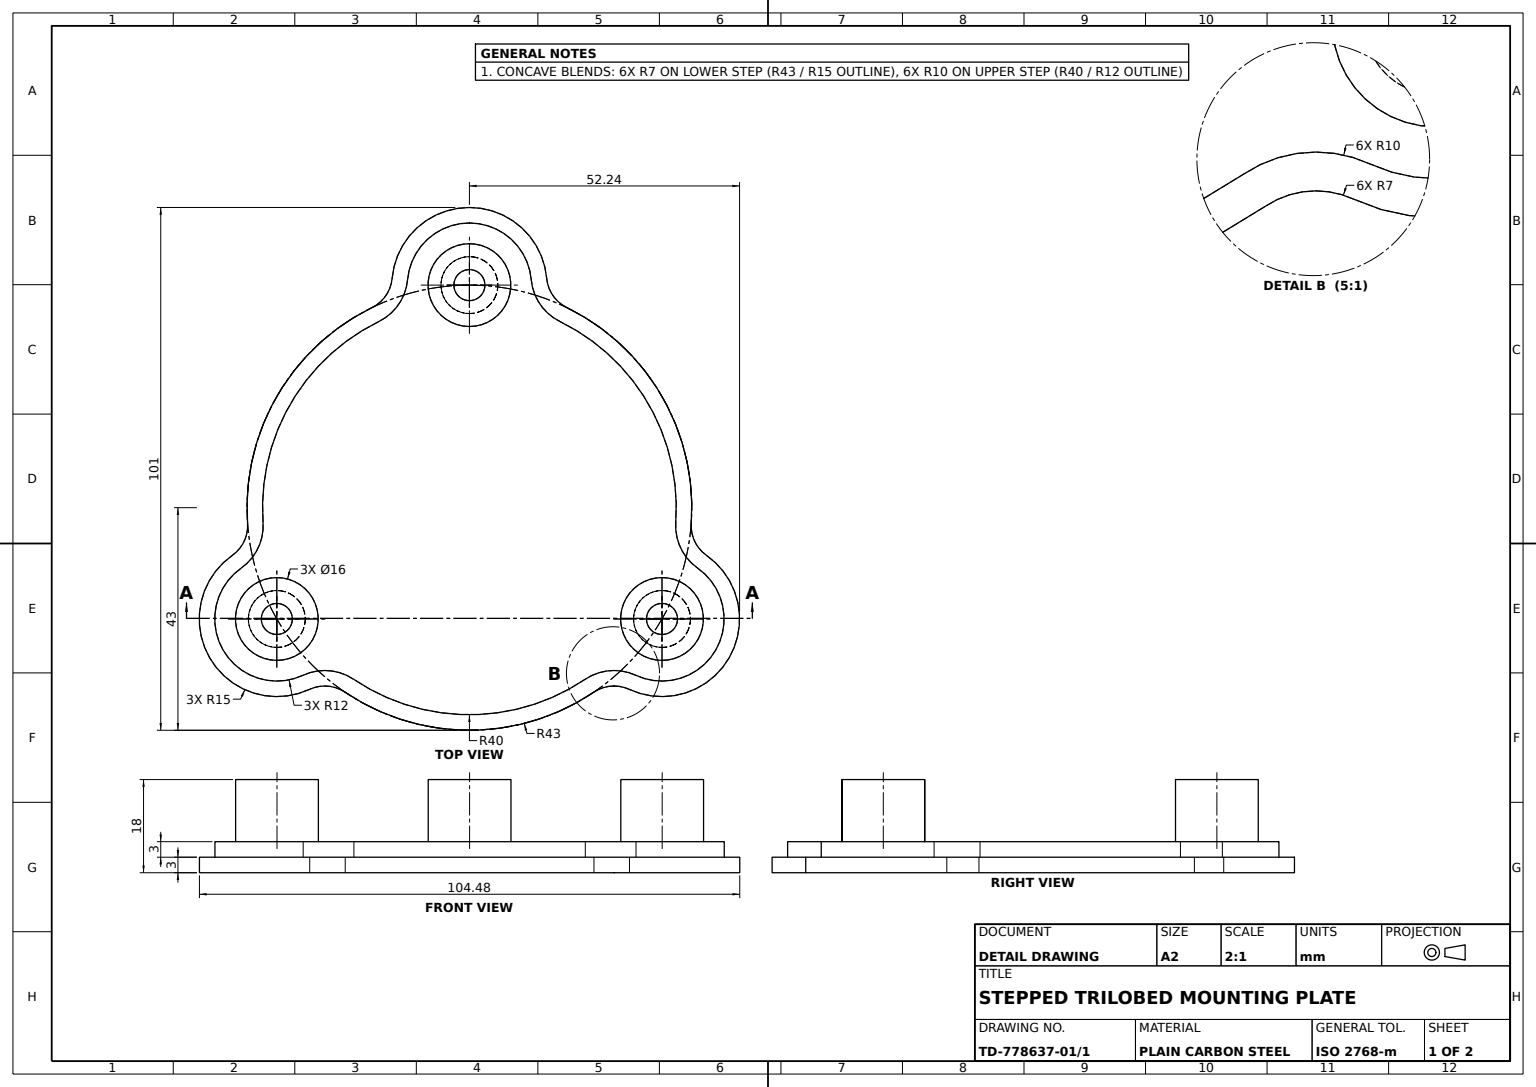
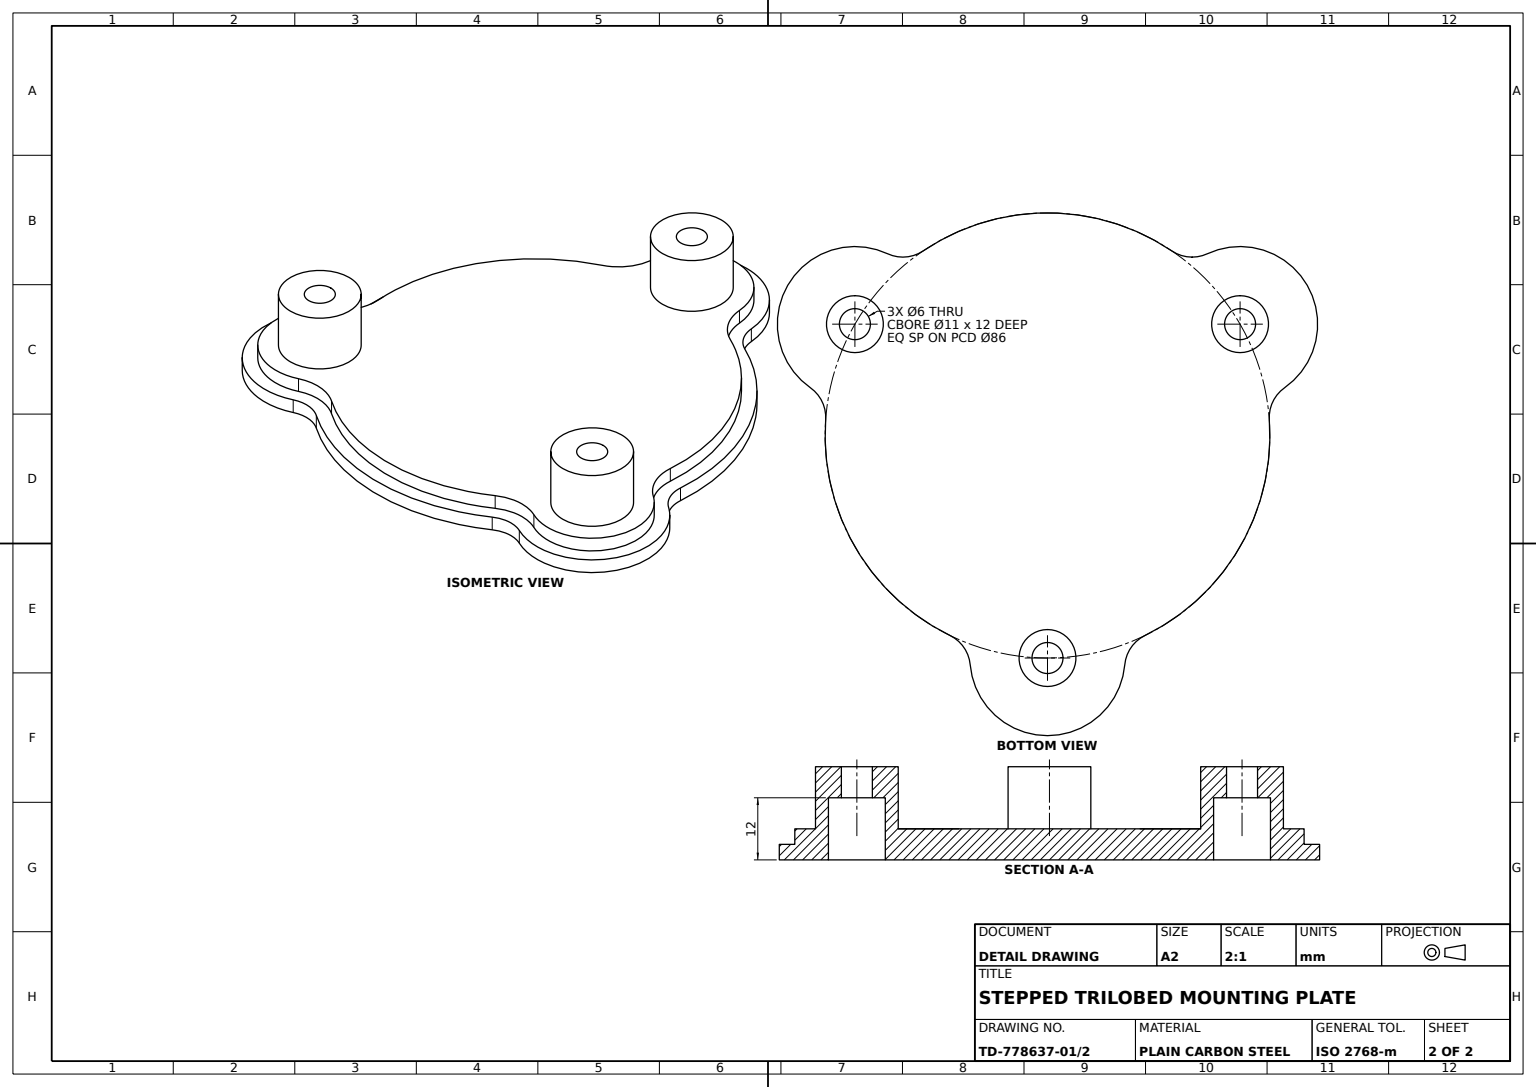
from build123d import *

# Parameters (mm, degrees)
BASE_FLANGE_PROFILE_R     = 8
BASE_FLANGE_3MM_DEPTH     = 3
RAISED_PLATE_3MM_DEPTH    = 3
LOBE_CUT_PROFILE_3X_R     = 8
LOBE_CUT_3X_13MM_DEPTH    = 13
BOSSES_3X_DEPTH           = 12
BOSSES_3X_DEPTH_BACK      = 6
BOSS_PROFILE_3X_R         = 8
BOSS_HOLE_PROFILE_3X_R    = 5.5
BOSS_HOLE_PROFILE_3X_R_2  = 3
BOSS_HOLES_3X_12MM_DEPTH  = 12
THROUGH_CUT_PROFILE_3X_R  = 3
THROUGH_CUT_3X_22MM_DEPTH = 22


with BuildPart() as part:
    # Base Flange Profile → Base Flange 3mm (new body)
    with BuildSketch(Plane(origin=(0, 0, 0), x_dir=(1, 0, 0), z_dir=(0, 1, 0))):
        with BuildLine():
            ThreePointArc((14.941453584, 44.323995772), (0, 58), (-14.941453584, 44.323995772))
            ThreePointArc((-14.941453584, 44.323995772), (-16.147655157, 40.973517523), (-18.846153454, 38.65))
            ThreePointArc((-18.846153454, 38.65), (-37.239092363, 21.5), (-42.894958583, -3.003752345))
            ThreePointArc((-42.894958583, -3.003752345), (-43.557934635, -6.502479184), (-45.856433127, -9.222319513))
            ThreePointArc((-45.856433127, -9.222319513), (-50.229473419, -29), (-30.914979544, -35.101676259))
            ThreePointArc((-30.914979544, -35.101676259), (-27.410279478, -34.471038339), (-24.048805129, -35.646247655))
            ThreePointArc((-24.048805129, -35.646247655), (0, -43), (24.048805129, -35.646247655))
            ThreePointArc((24.048805129, -35.646247655), (27.410279478, -34.471038339), (30.914979544, -35.101676259))
            ThreePointArc((30.914979544, -35.101676259), (50.229473419, -29), (45.856433127, -9.222319513))
            ThreePointArc((45.856433127, -9.222319513), (43.557934635, -6.502479184), (42.894958583, -3.003752345))
            ThreePointArc((42.894958583, -3.003752345), (37.239092363, 21.5), (18.846153454, 38.65))
            ThreePointArc((18.846153454, 38.65), (16.147655157, 40.973517523), (14.941453584, 44.323995772))
        make_face()
        with Locations(Location((0, 43, 0), (0, 0, 270))):
            Circle(BASE_FLANGE_PROFILE_R, mode=Mode.SUBTRACT)
        with Locations(Location((37.239092363, -21.5, 0), (0, 0, 270))):
            Circle(BASE_FLANGE_PROFILE_R, mode=Mode.SUBTRACT)
        with Locations(Location((-37.239092363, -21.5, 0), (0, 0, 270))):
            Circle(BASE_FLANGE_PROFILE_R, mode=Mode.SUBTRACT)
    extrude(amount=BASE_FLANGE_3MM_DEPTH)

    # Raised Plate Profile → Raised Plate 3mm (add)
    with BuildSketch(Plane(origin=(0, 3, 0), x_dir=(1, 0, 0), z_dir=(0, 1, 0))):
        with BuildLine():
            ThreePointArc((39.902287054, -2.794188228), (40.8493957, -7.792369426), (44.132964974, -11.67785561))
            ThreePointArc((44.132964974, -11.67785561), (47.631397208, -27.5), (32.179802107, -32.381341007))
            ThreePointArc((32.179802107, -32.381341007), (27.173087728, -31.480429693), (22.370981516, -33.159300144))
            ThreePointArc((22.370981516, -33.159300144), (0, -40), (-22.370981516, -33.159300144))
            ThreePointArc((-22.370981516, -33.159300144), (-27.173087728, -31.480429693), (-32.179802107, -32.381341007))
            ThreePointArc((-32.179802107, -32.381341007), (-47.631397208, -27.5), (-44.132964974, -11.67785561))
            ThreePointArc((-44.132964974, -11.67785561), (-40.8493957, -7.792369426), (-39.902287054, -2.794188228))
            ThreePointArc((-39.902287054, -2.794188228), (-34.641016151, 20), (-17.531305538, 35.953488372))
            ThreePointArc((-17.531305538, 35.953488372), (-13.676307972, 39.272799119), (-11.953162867, 44.059196617))
            ThreePointArc((-11.953162867, 44.059196617), (0, 55), (11.953162867, 44.059196617))
            ThreePointArc((11.953162867, 44.059196617), (13.676307972, 39.272799119), (17.531305538, 35.953488372))
            ThreePointArc((17.531305538, 35.953488372), (34.641016151, 20), (39.902287054, -2.794188228))
        make_face()
    extrude(amount=RAISED_PLATE_3MM_DEPTH)

    # Lobe Cut Profile 3x → Lobe Cut 3x 13mm (cut)
    with BuildSketch(Plane.XZ):
        with Locations(Location((0, -43, 0), (0, 0, 90))):
            Circle(LOBE_CUT_PROFILE_3X_R)
        with Locations(Location((37.239092363, 21.5, 0), (0, 0, 90))):
            Circle(LOBE_CUT_PROFILE_3X_R)
        with Locations(Location((-37.239092363, 21.5, 0), (0, 0, 90))):
            Circle(LOBE_CUT_PROFILE_3X_R)
    extrude(amount=-LOBE_CUT_3X_13MM_DEPTH, mode=Mode.SUBTRACT)

    # Boss Profile 3x → Bosses 3x (add, two sides: drawn at the far end of the back side and taken through both)
    with BuildSketch(Plane(origin=(0, 6, 0), x_dir=(1, 0, 0), z_dir=(0, 1, 0)).offset(-BOSSES_3X_DEPTH_BACK)):
        with Locations(Location((0, 43, 0), (0, 0, 270))):
            Circle(BOSS_PROFILE_3X_R)
        with Locations(Location((37.239092363, -21.5, 0), (0, 0, 270))):
            Circle(BOSS_PROFILE_3X_R)
        with Locations(Location((-37.239092363, -21.5, 0), (0, 0, 270))):
            Circle(BOSS_PROFILE_3X_R)
    extrude(amount=BOSSES_3X_DEPTH + BOSSES_3X_DEPTH_BACK)

    # Boss Hole Profile 3x → Boss Holes 3x 12mm (cut)
    # profile 1 of 3: a face of its own
    with BuildSketch(Plane.XZ):
        with Locations(Location((0, -43, 0), (0, 0, 270))):
            Circle(BOSS_HOLE_PROFILE_3X_R)
        with Locations(Location((0, -43, 0), (0, 0, 270))):
            Circle(BOSS_HOLE_PROFILE_3X_R_2, mode=Mode.SUBTRACT)
    # profile 2 of 3: a face of its own
    with BuildSketch(Plane.XZ):
        with Locations(Location((37.239092363, 21.5, 0), (0, 0, 270))):
            Circle(BOSS_HOLE_PROFILE_3X_R)
        with Locations(Location((37.239092363, 21.5, 0), (0, 0, 270))):
            Circle(BOSS_HOLE_PROFILE_3X_R_2, mode=Mode.SUBTRACT)
    # profile 3 of 3: a face of its own
    with BuildSketch(Plane.XZ):
        with Locations(Location((-37.239092363, 21.5, 0), (0, 0, 270))):
            Circle(BOSS_HOLE_PROFILE_3X_R)
        with Locations(Location((-37.239092363, 21.5, 0), (0, 0, 270))):
            Circle(BOSS_HOLE_PROFILE_3X_R_2, mode=Mode.SUBTRACT)
    extrude(amount=-BOSS_HOLES_3X_12MM_DEPTH, mode=Mode.SUBTRACT)

    # Through Cut Profile 3x → Through Cut 3x 22mm (cut)
    with BuildSketch(Plane.XZ):
        with Locations(Location((0, -43, 0), (0, 0, 270))):
            Circle(THROUGH_CUT_PROFILE_3X_R)
        with Locations(Location((37.239092363, 21.5, 0), (0, 0, 270))):
            Circle(THROUGH_CUT_PROFILE_3X_R)
        with Locations(Location((-37.239092363, 21.5, 0), (0, 0, 270))):
            Circle(THROUGH_CUT_PROFILE_3X_R)
    extrude(amount=-THROUGH_CUT_3X_22MM_DEPTH, mode=Mode.SUBTRACT)


solid = part.part
